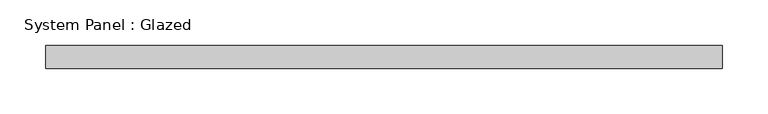
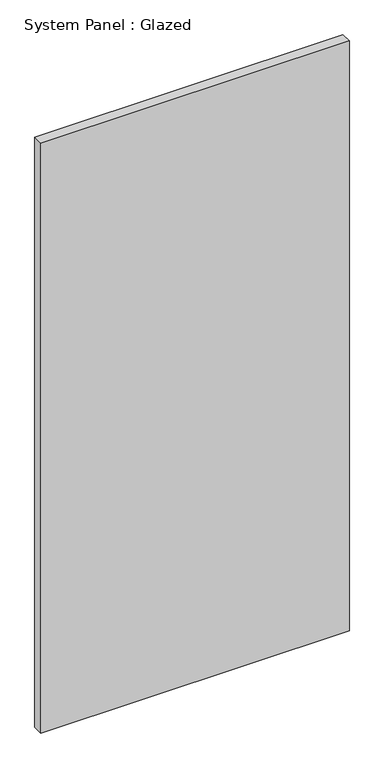
"""IFC4 building model written with IfcOpenShell, lengths in millimetres: plate geometry, System Panel : Glazed."""

from ifc_helpers import new_model, si_unit, origin, origin_with_axes, place, context, project, spatial, polyline, outline, extrude, source, transform, mapped, element, save


def system_panel_glazed_1c093cbc(model_context):
    return source(origin(), model_context, "Body", "SweptSolid", [
        extrude(outline(polyline([(371.475, 19.05), (-371.475, 19.05), (-371.475, 44.45), (371.475, 44.45), (371.475, 19.05)])), origin_with_axes(), (0.0, 0.0, 1.0), 1501.7655616),
    ])


if __name__ == "__main__":
    model = new_model("IFC4")
    model_context = context("Model", 3, world=origin())
    ifc_project = project(units=[si_unit("LENGTHUNIT", "METRE", prefix="MILLI")], contexts=[model_context])
    site = spatial("IfcSite", under=ifc_project)
    building = spatial("IfcBuilding", under=site)
    placement = place(None, origin())
    system_panel_glazed_shape = system_panel_glazed_1c093cbc(model_context)
    element("IfcPlate", 1, ObjectType="System Panel : Glazed", at=placement, inside=building, context=model_context, shape_type="MappedRepresentation", body=[
        mapped(system_panel_glazed_shape, transform((0.0, 0.0, 0.0), x_axis=(1.0, 0.0, 0.0), y_axis=(0.0, 1.0, 0.0), z_axis=(0.0, 0.0, 1.0))),
    ])
    save(model, "model.ifc")

# Revit data of these elements
# Type "System Panel : Glazed"
#   Construction Type Id = "GSP4R"
#   Analytic Construction = "1/8 in Pilkington single glazing"
#   Visual Light Transmittance = 0.9
#   Solar Heat Gain Coefficient = 0.86
#   Heat Transfer Coefficient (U) = 1.18115 BTU/(h·ft²·°F)
#   Define Thermal Properties by = 1
# Element 1 (IfcPlate, "System Panel : Glazed")
#   Materials on its faces: "Glass"
# Materials
#   "Glass": class "Glass", colour RGB 0 128 192, transparency 0.75, Description = "Soda Lime Glass", Cost = 0
